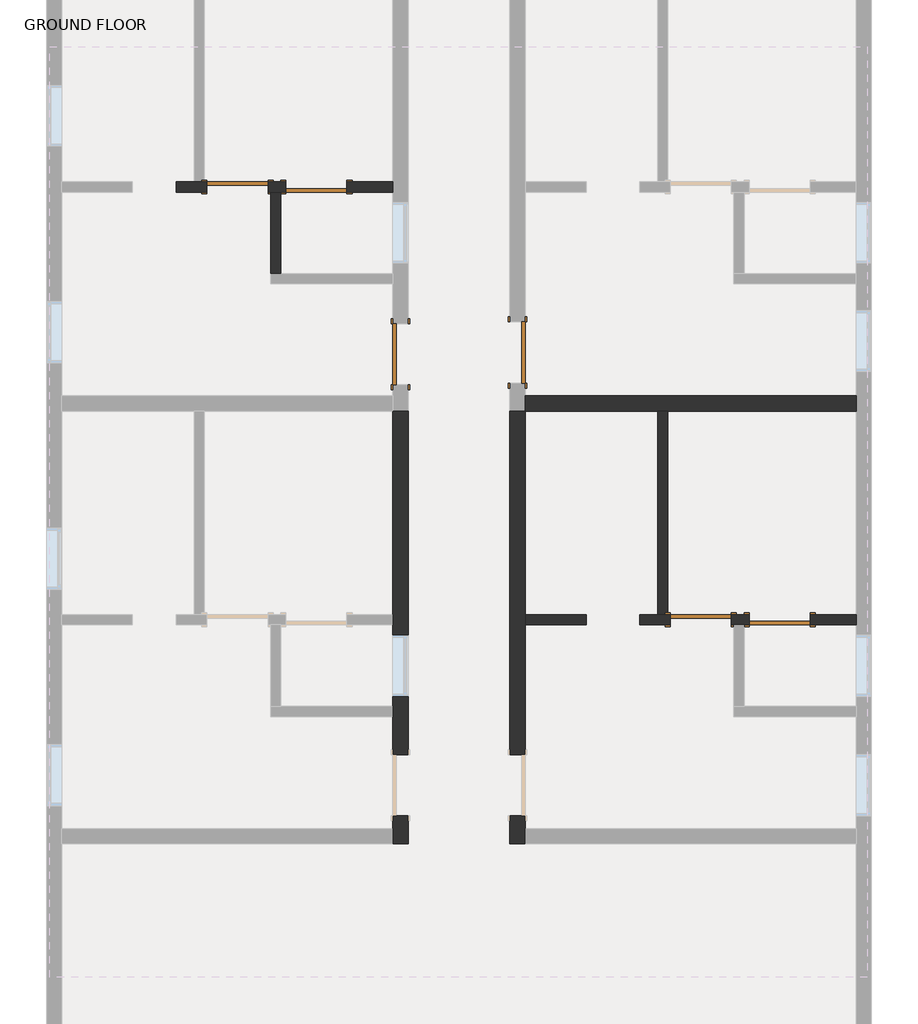
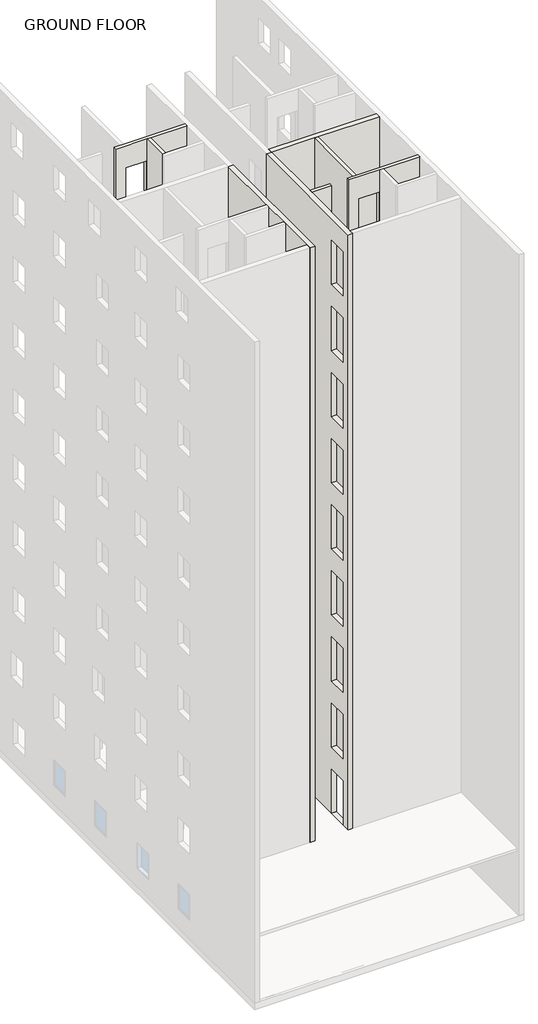
# One storey, part 3 of 7: 8 walls, 6 doors.
"""IFC4 building model written with IfcOpenShell, lengths in millimetres."""

from ifc_helpers import new_model, si_unit, origin, origin_with_axes, place, context, project, spatial, polyline, outline, extrude, faceted_brep, transform, mapped, element, save
from components import door_686f89d2, door_16372e1c, door_a90ba1ad, door_0ca8825f

model = new_model("IFC4")

# Units and contexts
model_context = context("Model", 3, world=origin())
ifc_project = project(units=[si_unit("LENGTHUNIT", "METRE", prefix="MILLI")], contexts=[model_context])

# Site, building, storey
site = spatial("IfcSite", under=ifc_project)
building = spatial("IfcBuilding", under=site)
storey = spatial("IfcBuildingStorey", under=building, Name="GROUND FLOOR", Elevation=0.0)

# Doors
placement = place(None, origin())
door_shape = door_686f89d2(model_context)
element("IfcDoor", 1, ObjectType="Single-Flush : 36\" x 84\"", at=placement, inside=storey, context=model_context, shape_type="MappedRepresentation", body=[
    mapped(door_shape, transform((-9863.5902461, -1001.7289408, 0.0), x_axis=(-1.0, 0.0, 0.0), y_axis=(0.0, -1.0, 0.0), z_axis=(0.0, 0.0, 1.0))),
])
element("IfcDoor", 2, ObjectType="Single-Flush : 36\" x 84\"", at=placement, inside=storey, context=model_context, shape_type="MappedRepresentation", body=[
    mapped(door_shape, transform((-2929.3902461, -7478.7289408, 0.0), x_axis=(-1.0, 0.0, 0.0), y_axis=(0.0, -1.0, 0.0), z_axis=(0.0, 0.0, 1.0))),
])
door_2_shape = door_16372e1c(model_context)
element("IfcDoor", 3, ObjectType="Single-Flush : 36\" x 84\"", at=placement, inside=storey, context=model_context, shape_type="MappedRepresentation", body=[
    mapped(door_2_shape, transform((-8682.4902461, -1001.7289408, 0.0), x_axis=(-1.0, 0.0, 0.0), y_axis=(0.0, -1.0, 0.0), z_axis=(0.0, 0.0, 1.0))),
])
element("IfcDoor", 4, ObjectType="Single-Flush : 36\" x 84\"", at=placement, inside=storey, context=model_context, shape_type="MappedRepresentation", body=[
    mapped(door_2_shape, transform((-1748.2902461, -7478.7289408, 0.0), x_axis=(-1.0, 0.0, 0.0), y_axis=(0.0, -1.0, 0.0), z_axis=(0.0, 0.0, 1.0))),
])
door_3_shape = door_a90ba1ad(model_context)
element("IfcDoor", 5, ObjectType="Single-Flush : 36\" x 84\"", at=placement, inside=storey, context=model_context, shape_type="MappedRepresentation", body=[
    mapped(door_3_shape, transform((-7425.1902461, -3503.6289408, 0.0), x_axis=(0.0, -1.0, 0.0), y_axis=(1.0, 0.0, 0.0), z_axis=(0.0, 0.0, 1.0))),
])
door_4_shape = door_0ca8825f(model_context)
element("IfcDoor", 6, ObjectType="Single-Flush : 36\" x 84\"", at=placement, inside=storey, context=model_context, shape_type="MappedRepresentation", body=[
    mapped(door_4_shape, transform((-5672.5902461, -3478.2289408, 0.0), x_axis=(0.0, -1.0, 0.0), y_axis=(1.0, 0.0, 0.0), z_axis=(0.0, 0.0, 1.0))),
])

# Walls
element("IfcWall", 7, ObjectType="Generic - 8\"", at=placement, inside=storey, context=model_context, shape_type="Brep", body=[
    faceted_brep([(-5558.2902461, -10831.5289408, 0.0), (-5558.2902461, -10602.9289408, 0.0), (-5558.2902461, -10412.4289408, 0.0), (-5558.2902461, -10412.4289408, 2133.6), (-5558.2902461, -9498.0289408, 2133.6), (-5558.2902461, -9498.0289408, 0.0), (-5558.2902461, -7554.9289408, 0.0), (-5558.2902461, -7402.5289408, 0.0), (-5558.2902461, -4354.5289408, 0.0), (-5558.2902461, -4354.5289408, 32004.0), (-5558.2902461, -7402.5289408, 32004.0), (-5558.2902461, -7554.9289408, 32004.0), (-5558.2902461, -10602.9289408, 32004.0), (-5558.2902461, -10831.5289408, 32004.0), (-5558.2902461, -9498.0289408, 3200.4), (-5558.2902461, -10412.4289408, 3200.4), (-5558.2902461, -10412.4289408, 5334.0), (-5558.2902461, -9498.0289408, 5334.0), (-5558.2902461, -9498.0289408, 6400.8), (-5558.2902461, -10412.4289408, 6400.8), (-5558.2902461, -10412.4289408, 8534.4), (-5558.2902461, -9498.0289408, 8534.4), (-5558.2902461, -9498.0289408, 9601.2), (-5558.2902461, -10412.4289408, 9601.2), (-5558.2902461, -10412.4289408, 11734.8), (-5558.2902461, -9498.0289408, 11734.8), (-5558.2902461, -9498.0289408, 12801.6), (-5558.2902461, -10412.4289408, 12801.6), (-5558.2902461, -10412.4289408, 14935.2), (-5558.2902461, -9498.0289408, 14935.2), (-5558.2902461, -9498.0289408, 16002.0), (-5558.2902461, -10412.4289408, 16002.0), (-5558.2902461, -10412.4289408, 18135.6), (-5558.2902461, -9498.0289408, 18135.6), (-5558.2902461, -9498.0289408, 19202.4), (-5558.2902461, -10412.4289408, 19202.4), (-5558.2902461, -10412.4289408, 21336.0), (-5558.2902461, -9498.0289408, 21336.0), (-5558.2902461, -9498.0289408, 22402.8), (-5558.2902461, -10412.4289408, 22402.8), (-5558.2902461, -10412.4289408, 24536.4), (-5558.2902461, -9498.0289408, 24536.4), (-5558.2902461, -9498.0289408, 25603.2), (-5558.2902461, -10412.4289408, 25603.2), (-5558.2902461, -10412.4289408, 27736.8), (-5558.2902461, -9498.0289408, 27736.8), (-5558.2902461, -9498.0289408, 28803.6), (-5558.2902461, -10412.4289408, 28803.6), (-5558.2902461, -10412.4289408, 30937.2), (-5558.2902461, -9498.0289408, 30937.2), (-5786.8902461, -10412.4289408, 2133.6), (-5786.8902461, -10412.4289408, 0.0), (-5786.8902461, -10831.5289408, 0.0), (-5786.8902461, -10831.5289408, 32004.0), (-5786.8902461, -4354.5289408, 32004.0), (-5786.8902461, -4354.5289408, 0.0), (-5786.8902461, -9498.0289408, 0.0), (-5786.8902461, -9498.0289408, 2133.6), (-5786.8902461, -9498.0289408, 3200.4), (-5786.8902461, -9498.0289408, 5334.0), (-5786.8902461, -10412.4289408, 5334.0), (-5786.8902461, -10412.4289408, 3200.4), (-5786.8902461, -9498.0289408, 6400.8), (-5786.8902461, -9498.0289408, 8534.4), (-5786.8902461, -10412.4289408, 8534.4), (-5786.8902461, -10412.4289408, 6400.8), (-5786.8902461, -9498.0289408, 9601.2), (-5786.8902461, -9498.0289408, 11734.8), (-5786.8902461, -10412.4289408, 11734.8), (-5786.8902461, -10412.4289408, 9601.2), (-5786.8902461, -9498.0289408, 12801.6), (-5786.8902461, -9498.0289408, 14935.2), (-5786.8902461, -10412.4289408, 14935.2), (-5786.8902461, -10412.4289408, 12801.6), (-5786.8902461, -9498.0289408, 16002.0), (-5786.8902461, -9498.0289408, 18135.6), (-5786.8902461, -10412.4289408, 18135.6), (-5786.8902461, -10412.4289408, 16002.0), (-5786.8902461, -9498.0289408, 19202.4), (-5786.8902461, -9498.0289408, 21336.0), (-5786.8902461, -10412.4289408, 21336.0), (-5786.8902461, -10412.4289408, 19202.4), (-5786.8902461, -9498.0289408, 22402.8), (-5786.8902461, -9498.0289408, 24536.4), (-5786.8902461, -10412.4289408, 24536.4), (-5786.8902461, -10412.4289408, 22402.8), (-5786.8902461, -9498.0289408, 25603.2), (-5786.8902461, -9498.0289408, 27736.8), (-5786.8902461, -10412.4289408, 27736.8), (-5786.8902461, -10412.4289408, 25603.2), (-5786.8902461, -9498.0289408, 28803.6), (-5786.8902461, -9498.0289408, 30937.2), (-5786.8902461, -10412.4289408, 30937.2), (-5786.8902461, -10412.4289408, 28803.6)], [[[0, 1, 2, 3, 4, 5, 6, 7, 8, 9, 10, 11, 12, 13], [14, 15, 16, 17], [18, 19, 20, 21], [22, 23, 24, 25], [26, 27, 28, 29], [30, 31, 32, 33], [34, 35, 36, 37], [38, 39, 40, 41], [42, 43, 44, 45], [46, 47, 48, 49]], [[50, 51, 52, 53, 54, 55, 56, 57], [58, 59, 60, 61], [62, 63, 64, 65], [66, 67, 68, 69], [70, 71, 72, 73], [74, 75, 76, 77], [78, 79, 80, 81], [82, 83, 84, 85], [86, 87, 88, 89], [90, 91, 92, 93]], [[56, 55, 8, 7, 6, 5]], [[52, 51, 2, 1, 0]], [[13, 12, 11, 10, 9, 54, 53]], [[0, 13, 53, 52]], [[9, 8, 55, 54]], [[3, 2, 51, 50]], [[4, 3, 50, 57]], [[5, 4, 57, 56]], [[15, 14, 58, 61]], [[16, 15, 61, 60]], [[17, 16, 60, 59]], [[14, 17, 59, 58]], [[19, 18, 62, 65]], [[20, 19, 65, 64]], [[21, 20, 64, 63]], [[18, 21, 63, 62]], [[23, 22, 66, 69]], [[24, 23, 69, 68]], [[25, 24, 68, 67]], [[22, 25, 67, 66]], [[27, 26, 70, 73]], [[28, 27, 73, 72]], [[29, 28, 72, 71]], [[26, 29, 71, 70]], [[31, 30, 74, 77]], [[32, 31, 77, 76]], [[33, 32, 76, 75]], [[30, 33, 75, 74]], [[35, 34, 78, 81]], [[36, 35, 81, 80]], [[37, 36, 80, 79]], [[34, 37, 79, 78]], [[39, 38, 82, 85]], [[40, 39, 85, 84]], [[41, 40, 84, 83]], [[38, 41, 83, 82]], [[43, 42, 86, 89]], [[44, 43, 89, 88]], [[45, 44, 88, 87]], [[42, 45, 87, 86]], [[47, 46, 90, 93]], [[48, 47, 93, 92]], [[49, 48, 92, 91]], [[46, 49, 91, 90]]]),
])
element("IfcWall", 8, ObjectType="INNER WALL 2", at=placement, inside=storey, context=model_context, shape_type="Brep", body=[
    faceted_brep([(-2472.1902461, -7554.9289408, 0.0), (-2434.0902461, -7554.9289408, 0.0), (-2281.6902461, -7554.9289408, 0.0), (-2205.4902461, -7554.9289408, 0.0), (-2205.4902461, -7554.9289408, 2133.6), (-1291.0902461, -7554.9289408, 2133.6), (-1291.0902461, -7554.9289408, 0.0), (-605.2902461, -7554.9289408, 0.0), (-605.2902461, -7554.9289408, 32004.0), (-2281.6902461, -7554.9289408, 32004.0), (-2434.0902461, -7554.9289408, 32004.0), (-3843.7902461, -7554.9289408, 32004.0), (-3843.7902461, -7554.9289408, 0.0), (-3386.5902461, -7554.9289408, 0.0), (-3386.5902461, -7554.9289408, 2133.6), (-2472.1902461, -7554.9289408, 2133.6), (-2472.1902461, -7554.9289408, 3200.4), (-3386.5902461, -7554.9289408, 3200.4), (-3386.5902461, -7554.9289408, 5334.0), (-2472.1902461, -7554.9289408, 5334.0), (-1291.0902461, -7554.9289408, 3200.4), (-2205.4902461, -7554.9289408, 3200.4), (-2205.4902461, -7554.9289408, 5334.0), (-1291.0902461, -7554.9289408, 5334.0), (-2472.1902461, -7554.9289408, 6400.8), (-3386.5902461, -7554.9289408, 6400.8), (-3386.5902461, -7554.9289408, 8534.4), (-2472.1902461, -7554.9289408, 8534.4), (-1291.0902461, -7554.9289408, 6400.8), (-2205.4902461, -7554.9289408, 6400.8), (-2205.4902461, -7554.9289408, 8534.4), (-1291.0902461, -7554.9289408, 8534.4), (-2472.1902461, -7554.9289408, 9601.2), (-3386.5902461, -7554.9289408, 9601.2), (-3386.5902461, -7554.9289408, 11734.8), (-2472.1902461, -7554.9289408, 11734.8), (-1291.0902461, -7554.9289408, 9601.2), (-2205.4902461, -7554.9289408, 9601.2), (-2205.4902461, -7554.9289408, 11734.8), (-1291.0902461, -7554.9289408, 11734.8), (-1291.0902461, -7554.9289408, 12801.6), (-2205.4902461, -7554.9289408, 12801.6), (-2205.4902461, -7554.9289408, 14935.2), (-1291.0902461, -7554.9289408, 14935.2), (-3386.5902461, -7554.9289408, 12801.6), (-3386.5902461, -7554.9289408, 14935.2), (-2472.1902461, -7554.9289408, 14935.2), (-2472.1902461, -7554.9289408, 12801.6), (-2472.1902461, -7554.9289408, 16002.0), (-3386.5902461, -7554.9289408, 16002.0), (-3386.5902461, -7554.9289408, 18135.6), (-2472.1902461, -7554.9289408, 18135.6), (-1291.0902461, -7554.9289408, 16002.0), (-2205.4902461, -7554.9289408, 16002.0), (-2205.4902461, -7554.9289408, 18135.6), (-1291.0902461, -7554.9289408, 18135.6), (-1291.0902461, -7554.9289408, 19202.4), (-2205.4902461, -7554.9289408, 19202.4), (-2205.4902461, -7554.9289408, 21336.0), (-1291.0902461, -7554.9289408, 21336.0), (-2472.1902461, -7554.9289408, 19202.4), (-3386.5902461, -7554.9289408, 19202.4), (-3386.5902461, -7554.9289408, 21336.0), (-2472.1902461, -7554.9289408, 21336.0), (-1291.0902461, -7554.9289408, 22402.8), (-2205.4902461, -7554.9289408, 22402.8), (-2205.4902461, -7554.9289408, 24536.4), (-1291.0902461, -7554.9289408, 24536.4), (-2472.1902461, -7554.9289408, 22402.8), (-3386.5902461, -7554.9289408, 22402.8), (-3386.5902461, -7554.9289408, 24536.4), (-2472.1902461, -7554.9289408, 24536.4), (-2472.1902461, -7554.9289408, 28803.6), (-3386.5902461, -7554.9289408, 28803.6), (-3386.5902461, -7554.9289408, 30937.2), (-2472.1902461, -7554.9289408, 30937.2), (-1291.0902461, -7554.9289408, 28803.6), (-2205.4902461, -7554.9289408, 28803.6), (-2205.4902461, -7554.9289408, 30937.2), (-1291.0902461, -7554.9289408, 30937.2), (-2205.4902461, -7402.5289408, 2133.6), (-2205.4902461, -7402.5289408, 0.0), (-2472.1902461, -7402.5289408, 0.0), (-2472.1902461, -7402.5289408, 2133.6), (-3386.5902461, -7402.5289408, 2133.6), (-3386.5902461, -7402.5289408, 0.0), (-3424.6902461, -7402.5289408, 0.0), (-3577.0902461, -7402.5289408, 0.0), (-3843.7902461, -7402.5289408, 0.0), (-3843.7902461, -7402.5289408, 32004.0), (-3577.0902461, -7402.5289408, 32004.0), (-3424.6902461, -7402.5289408, 32004.0), (-605.2902461, -7402.5289408, 32004.0), (-605.2902461, -7402.5289408, 0.0), (-1291.0902461, -7402.5289408, 0.0), (-1291.0902461, -7402.5289408, 2133.6), (-2472.1902461, -7402.5289408, 3200.4), (-2472.1902461, -7402.5289408, 5334.0), (-3386.5902461, -7402.5289408, 5334.0), (-3386.5902461, -7402.5289408, 3200.4), (-1291.0902461, -7402.5289408, 3200.4), (-1291.0902461, -7402.5289408, 5334.0), (-2205.4902461, -7402.5289408, 5334.0), (-2205.4902461, -7402.5289408, 3200.4), (-2472.1902461, -7402.5289408, 6400.8), (-2472.1902461, -7402.5289408, 8534.4), (-3386.5902461, -7402.5289408, 8534.4), (-3386.5902461, -7402.5289408, 6400.8), (-1291.0902461, -7402.5289408, 6400.8), (-1291.0902461, -7402.5289408, 8534.4), (-2205.4902461, -7402.5289408, 8534.4), (-2205.4902461, -7402.5289408, 6400.8), (-2472.1902461, -7402.5289408, 9601.2), (-2472.1902461, -7402.5289408, 11734.8), (-3386.5902461, -7402.5289408, 11734.8), (-3386.5902461, -7402.5289408, 9601.2), (-1291.0902461, -7402.5289408, 9601.2), (-1291.0902461, -7402.5289408, 11734.8), (-2205.4902461, -7402.5289408, 11734.8), (-2205.4902461, -7402.5289408, 9601.2), (-1291.0902461, -7402.5289408, 12801.6), (-1291.0902461, -7402.5289408, 14935.2), (-2205.4902461, -7402.5289408, 14935.2), (-2205.4902461, -7402.5289408, 12801.6), (-3386.5902461, -7402.5289408, 12801.6), (-2472.1902461, -7402.5289408, 12801.6), (-2472.1902461, -7402.5289408, 14935.2), (-3386.5902461, -7402.5289408, 14935.2), (-2472.1902461, -7402.5289408, 16002.0), (-2472.1902461, -7402.5289408, 18135.6), (-3386.5902461, -7402.5289408, 18135.6), (-3386.5902461, -7402.5289408, 16002.0), (-1291.0902461, -7402.5289408, 16002.0), (-1291.0902461, -7402.5289408, 18135.6), (-2205.4902461, -7402.5289408, 18135.6), (-2205.4902461, -7402.5289408, 16002.0), (-1291.0902461, -7402.5289408, 19202.4), (-1291.0902461, -7402.5289408, 21336.0), (-2205.4902461, -7402.5289408, 21336.0), (-2205.4902461, -7402.5289408, 19202.4), (-2472.1902461, -7402.5289408, 19202.4), (-2472.1902461, -7402.5289408, 21336.0), (-3386.5902461, -7402.5289408, 21336.0), (-3386.5902461, -7402.5289408, 19202.4), (-1291.0902461, -7402.5289408, 22402.8), (-1291.0902461, -7402.5289408, 24536.4), (-2205.4902461, -7402.5289408, 24536.4), (-2205.4902461, -7402.5289408, 22402.8), (-2472.1902461, -7402.5289408, 22402.8), (-2472.1902461, -7402.5289408, 24536.4), (-3386.5902461, -7402.5289408, 24536.4), (-3386.5902461, -7402.5289408, 22402.8), (-2472.1902461, -7402.5289408, 28803.6), (-2472.1902461, -7402.5289408, 30937.2), (-3386.5902461, -7402.5289408, 30937.2), (-3386.5902461, -7402.5289408, 28803.6), (-1291.0902461, -7402.5289408, 28803.6), (-1291.0902461, -7402.5289408, 30937.2), (-2205.4902461, -7402.5289408, 30937.2), (-2205.4902461, -7402.5289408, 28803.6)], [[[0, 1, 2, 3, 4, 5, 6, 7, 8, 9, 10, 11, 12, 13, 14, 15], [16, 17, 18, 19], [20, 21, 22, 23], [24, 25, 26, 27], [28, 29, 30, 31], [32, 33, 34, 35], [36, 37, 38, 39], [40, 41, 42, 43], [44, 45, 46, 47], [48, 49, 50, 51], [52, 53, 54, 55], [56, 57, 58, 59], [60, 61, 62, 63], [64, 65, 66, 67], [68, 69, 70, 71], [72, 73, 74, 75], [76, 77, 78, 79]], [[80, 81, 82, 83, 84, 85, 86, 87, 88, 89, 90, 91, 92, 93, 94, 95], [96, 97, 98, 99], [100, 101, 102, 103], [104, 105, 106, 107], [108, 109, 110, 111], [112, 113, 114, 115], [116, 117, 118, 119], [120, 121, 122, 123], [124, 125, 126, 127], [128, 129, 130, 131], [132, 133, 134, 135], [136, 137, 138, 139], [140, 141, 142, 143], [144, 145, 146, 147], [148, 149, 150, 151], [152, 153, 154, 155], [156, 157, 158, 159]], [[88, 87, 86, 85, 13, 12]], [[94, 93, 7, 6]], [[82, 81, 3, 2, 1, 0]], [[11, 10, 9, 8, 92, 91, 90, 89]], [[12, 11, 89, 88]], [[8, 7, 93, 92]], [[14, 13, 85, 84]], [[15, 14, 84, 83]], [[0, 15, 83, 82]], [[4, 3, 81, 80]], [[5, 4, 80, 95]], [[6, 5, 95, 94]], [[17, 16, 96, 99]], [[18, 17, 99, 98]], [[19, 18, 98, 97]], [[16, 19, 97, 96]], [[21, 20, 100, 103]], [[22, 21, 103, 102]], [[23, 22, 102, 101]], [[20, 23, 101, 100]], [[25, 24, 104, 107]], [[26, 25, 107, 106]], [[27, 26, 106, 105]], [[24, 27, 105, 104]], [[29, 28, 108, 111]], [[30, 29, 111, 110]], [[31, 30, 110, 109]], [[28, 31, 109, 108]], [[33, 32, 112, 115]], [[34, 33, 115, 114]], [[35, 34, 114, 113]], [[32, 35, 113, 112]], [[37, 36, 116, 119]], [[38, 37, 119, 118]], [[39, 38, 118, 117]], [[36, 39, 117, 116]], [[41, 40, 120, 123]], [[42, 41, 123, 122]], [[43, 42, 122, 121]], [[40, 43, 121, 120]], [[125, 124, 44, 47]], [[126, 125, 47, 46]], [[127, 126, 46, 45]], [[124, 127, 45, 44]], [[49, 48, 128, 131]], [[50, 49, 131, 130]], [[51, 50, 130, 129]], [[48, 51, 129, 128]], [[53, 52, 132, 135]], [[54, 53, 135, 134]], [[55, 54, 134, 133]], [[52, 55, 133, 132]], [[57, 56, 136, 139]], [[58, 57, 139, 138]], [[59, 58, 138, 137]], [[56, 59, 137, 136]], [[61, 60, 140, 143]], [[62, 61, 143, 142]], [[63, 62, 142, 141]], [[60, 63, 141, 140]], [[65, 64, 144, 147]], [[66, 65, 147, 146]], [[67, 66, 146, 145]], [[64, 67, 145, 144]], [[69, 68, 148, 151]], [[70, 69, 151, 150]], [[71, 70, 150, 149]], [[68, 71, 149, 148]], [[73, 72, 152, 155]], [[74, 73, 155, 154]], [[75, 74, 154, 153]], [[72, 75, 153, 152]], [[77, 76, 156, 159]], [[78, 77, 159, 158]], [[79, 78, 158, 157]], [[76, 79, 157, 156]]]),
])
element("IfcWall", 9, ObjectType="INNER WALL 2", at=placement, inside=storey, context=model_context, shape_type="SweptSolid", body=[
    extrude(outline(polyline([(-3424.6902461, -4354.5289408), (-3424.6902461, -7402.5289408), (-3577.0902461, -7402.5289408), (-3577.0902461, -4354.5289408), (-3424.6902461, -4354.5289408)])), origin_with_axes(), (0.0, 0.0, 1.0), 32004.0),
])
element("IfcWall", 10, ObjectType="INNER WALL 2", at=placement, inside=storey, context=model_context, shape_type="Brep", body=[
    faceted_brep([(-9406.3902461, -1077.9289408, 0.0), (-9368.2902461, -1077.9289408, 0.0), (-9215.8902461, -1077.9289408, 0.0), (-9139.6902461, -1077.9289408, 0.0), (-9139.6902461, -1077.9289408, 2133.6), (-8225.2902461, -1077.9289408, 2133.6), (-8225.2902461, -1077.9289408, 0.0), (-7539.4902461, -1077.9289408, 0.0), (-7539.4902461, -1077.9289408, 32004.0), (-9215.8902461, -1077.9289408, 32004.0), (-9368.2902461, -1077.9289408, 32004.0), (-10777.9902461, -1077.9289408, 32004.0), (-10777.9902461, -1077.9289408, 0.0), (-10320.7902461, -1077.9289408, 0.0), (-10320.7902461, -1077.9289408, 2133.6), (-9406.3902461, -1077.9289408, 2133.6), (-9406.3902461, -1077.9289408, 3200.4), (-10320.7902461, -1077.9289408, 3200.4), (-10320.7902461, -1077.9289408, 5334.0), (-9406.3902461, -1077.9289408, 5334.0), (-8225.2902461, -1077.9289408, 3200.4), (-9139.6902461, -1077.9289408, 3200.4), (-9139.6902461, -1077.9289408, 5334.0), (-8225.2902461, -1077.9289408, 5334.0), (-8225.2902461, -1077.9289408, 6400.8), (-9139.6902461, -1077.9289408, 6400.8), (-9139.6902461, -1077.9289408, 8534.4), (-8225.2902461, -1077.9289408, 8534.4), (-9406.3902461, -1077.9289408, 6400.8), (-10320.7902461, -1077.9289408, 6400.8), (-10320.7902461, -1077.9289408, 8534.4), (-9406.3902461, -1077.9289408, 8534.4), (-9406.3902461, -1077.9289408, 9601.2), (-10320.7902461, -1077.9289408, 9601.2), (-10320.7902461, -1077.9289408, 11734.8), (-9406.3902461, -1077.9289408, 11734.8), (-8225.2902461, -1077.9289408, 9601.2), (-9139.6902461, -1077.9289408, 9601.2), (-9139.6902461, -1077.9289408, 11734.8), (-8225.2902461, -1077.9289408, 11734.8), (-9406.3902461, -1077.9289408, 12801.6), (-10320.7902461, -1077.9289408, 12801.6), (-10320.7902461, -1077.9289408, 14935.2), (-9406.3902461, -1077.9289408, 14935.2), (-8225.2902461, -1077.9289408, 12801.6), (-9139.6902461, -1077.9289408, 12801.6), (-9139.6902461, -1077.9289408, 14935.2), (-8225.2902461, -1077.9289408, 14935.2), (-9406.3902461, -1077.9289408, 16002.0), (-10320.7902461, -1077.9289408, 16002.0), (-10320.7902461, -1077.9289408, 18135.6), (-9406.3902461, -1077.9289408, 18135.6), (-8225.2902461, -1077.9289408, 16002.0), (-9139.6902461, -1077.9289408, 16002.0), (-9139.6902461, -1077.9289408, 18135.6), (-8225.2902461, -1077.9289408, 18135.6), (-9406.3902461, -1077.9289408, 19202.4), (-10320.7902461, -1077.9289408, 19202.4), (-10320.7902461, -1077.9289408, 21336.0), (-9406.3902461, -1077.9289408, 21336.0), (-8225.2902461, -1077.9289408, 19202.4), (-9139.6902461, -1077.9289408, 19202.4), (-9139.6902461, -1077.9289408, 21336.0), (-8225.2902461, -1077.9289408, 21336.0), (-9406.3902461, -1077.9289408, 22402.8), (-10320.7902461, -1077.9289408, 22402.8), (-10320.7902461, -1077.9289408, 24536.4), (-9406.3902461, -1077.9289408, 24536.4), (-8225.2902461, -1077.9289408, 22402.8), (-9139.6902461, -1077.9289408, 22402.8), (-9139.6902461, -1077.9289408, 24536.4), (-8225.2902461, -1077.9289408, 24536.4), (-8225.2902461, -1077.9289408, 25603.2), (-9139.6902461, -1077.9289408, 25603.2), (-9139.6902461, -1077.9289408, 27736.8), (-8225.2902461, -1077.9289408, 27736.8), (-9406.3902461, -1077.9289408, 25603.2), (-10320.7902461, -1077.9289408, 25603.2), (-10320.7902461, -1077.9289408, 27736.8), (-9406.3902461, -1077.9289408, 27736.8), (-9406.3902461, -1077.9289408, 28803.6), (-10320.7902461, -1077.9289408, 28803.6), (-10320.7902461, -1077.9289408, 30937.2), (-9406.3902461, -1077.9289408, 30937.2), (-8225.2902461, -1077.9289408, 28803.6), (-9139.6902461, -1077.9289408, 28803.6), (-9139.6902461, -1077.9289408, 30937.2), (-8225.2902461, -1077.9289408, 30937.2), (-9139.6902461, -925.5289408, 2133.6), (-9139.6902461, -925.5289408, 0.0), (-9406.3902461, -925.5289408, 0.0), (-9406.3902461, -925.5289408, 2133.6), (-10320.7902461, -925.5289408, 2133.6), (-10320.7902461, -925.5289408, 0.0), (-10358.8902461, -925.5289408, 0.0), (-10511.2902461, -925.5289408, 0.0), (-10777.9902461, -925.5289408, 0.0), (-10777.9902461, -925.5289408, 32004.0), (-10511.2902461, -925.5289408, 32004.0), (-10358.8902461, -925.5289408, 32004.0), (-7539.4902461, -925.5289408, 32004.0), (-7539.4902461, -925.5289408, 0.0), (-8225.2902461, -925.5289408, 0.0), (-8225.2902461, -925.5289408, 2133.6), (-9406.3902461, -925.5289408, 3200.4), (-9406.3902461, -925.5289408, 5334.0), (-10320.7902461, -925.5289408, 5334.0), (-10320.7902461, -925.5289408, 3200.4), (-8225.2902461, -925.5289408, 3200.4), (-8225.2902461, -925.5289408, 5334.0), (-9139.6902461, -925.5289408, 5334.0), (-9139.6902461, -925.5289408, 3200.4), (-8225.2902461, -925.5289408, 6400.8), (-8225.2902461, -925.5289408, 8534.4), (-9139.6902461, -925.5289408, 8534.4), (-9139.6902461, -925.5289408, 6400.8), (-9406.3902461, -925.5289408, 6400.8), (-9406.3902461, -925.5289408, 8534.4), (-10320.7902461, -925.5289408, 8534.4), (-10320.7902461, -925.5289408, 6400.8), (-9406.3902461, -925.5289408, 9601.2), (-9406.3902461, -925.5289408, 11734.8), (-10320.7902461, -925.5289408, 11734.8), (-10320.7902461, -925.5289408, 9601.2), (-8225.2902461, -925.5289408, 9601.2), (-8225.2902461, -925.5289408, 11734.8), (-9139.6902461, -925.5289408, 11734.8), (-9139.6902461, -925.5289408, 9601.2), (-9406.3902461, -925.5289408, 12801.6), (-9406.3902461, -925.5289408, 14935.2), (-10320.7902461, -925.5289408, 14935.2), (-10320.7902461, -925.5289408, 12801.6), (-8225.2902461, -925.5289408, 12801.6), (-8225.2902461, -925.5289408, 14935.2), (-9139.6902461, -925.5289408, 14935.2), (-9139.6902461, -925.5289408, 12801.6), (-9406.3902461, -925.5289408, 16002.0), (-9406.3902461, -925.5289408, 18135.6), (-10320.7902461, -925.5289408, 18135.6), (-10320.7902461, -925.5289408, 16002.0), (-8225.2902461, -925.5289408, 16002.0), (-8225.2902461, -925.5289408, 18135.6), (-9139.6902461, -925.5289408, 18135.6), (-9139.6902461, -925.5289408, 16002.0), (-9406.3902461, -925.5289408, 19202.4), (-9406.3902461, -925.5289408, 21336.0), (-10320.7902461, -925.5289408, 21336.0), (-10320.7902461, -925.5289408, 19202.4), (-8225.2902461, -925.5289408, 19202.4), (-8225.2902461, -925.5289408, 21336.0), (-9139.6902461, -925.5289408, 21336.0), (-9139.6902461, -925.5289408, 19202.4), (-9406.3902461, -925.5289408, 22402.8), (-9406.3902461, -925.5289408, 24536.4), (-10320.7902461, -925.5289408, 24536.4), (-10320.7902461, -925.5289408, 22402.8), (-8225.2902461, -925.5289408, 22402.8), (-8225.2902461, -925.5289408, 24536.4), (-9139.6902461, -925.5289408, 24536.4), (-9139.6902461, -925.5289408, 22402.8), (-8225.2902461, -925.5289408, 25603.2), (-8225.2902461, -925.5289408, 27736.8), (-9139.6902461, -925.5289408, 27736.8), (-9139.6902461, -925.5289408, 25603.2), (-9406.3902461, -925.5289408, 25603.2), (-9406.3902461, -925.5289408, 27736.8), (-10320.7902461, -925.5289408, 27736.8), (-10320.7902461, -925.5289408, 25603.2), (-9406.3902461, -925.5289408, 28803.6), (-9406.3902461, -925.5289408, 30937.2), (-10320.7902461, -925.5289408, 30937.2), (-10320.7902461, -925.5289408, 28803.6), (-8225.2902461, -925.5289408, 28803.6), (-8225.2902461, -925.5289408, 30937.2), (-9139.6902461, -925.5289408, 30937.2), (-9139.6902461, -925.5289408, 28803.6)], [[[0, 1, 2, 3, 4, 5, 6, 7, 8, 9, 10, 11, 12, 13, 14, 15], [16, 17, 18, 19], [20, 21, 22, 23], [24, 25, 26, 27], [28, 29, 30, 31], [32, 33, 34, 35], [36, 37, 38, 39], [40, 41, 42, 43], [44, 45, 46, 47], [48, 49, 50, 51], [52, 53, 54, 55], [56, 57, 58, 59], [60, 61, 62, 63], [64, 65, 66, 67], [68, 69, 70, 71], [72, 73, 74, 75], [76, 77, 78, 79], [80, 81, 82, 83], [84, 85, 86, 87]], [[88, 89, 90, 91, 92, 93, 94, 95, 96, 97, 98, 99, 100, 101, 102, 103], [104, 105, 106, 107], [108, 109, 110, 111], [112, 113, 114, 115], [116, 117, 118, 119], [120, 121, 122, 123], [124, 125, 126, 127], [128, 129, 130, 131], [132, 133, 134, 135], [136, 137, 138, 139], [140, 141, 142, 143], [144, 145, 146, 147], [148, 149, 150, 151], [152, 153, 154, 155], [156, 157, 158, 159], [160, 161, 162, 163], [164, 165, 166, 167], [168, 169, 170, 171], [172, 173, 174, 175]], [[96, 95, 94, 93, 13, 12]], [[102, 101, 7, 6]], [[90, 89, 3, 2, 1, 0]], [[11, 10, 9, 8, 100, 99, 98, 97]], [[12, 11, 97, 96]], [[8, 7, 101, 100]], [[14, 13, 93, 92]], [[15, 14, 92, 91]], [[0, 15, 91, 90]], [[4, 3, 89, 88]], [[5, 4, 88, 103]], [[6, 5, 103, 102]], [[17, 16, 104, 107]], [[18, 17, 107, 106]], [[19, 18, 106, 105]], [[16, 19, 105, 104]], [[21, 20, 108, 111]], [[22, 21, 111, 110]], [[23, 22, 110, 109]], [[20, 23, 109, 108]], [[25, 24, 112, 115]], [[26, 25, 115, 114]], [[27, 26, 114, 113]], [[24, 27, 113, 112]], [[29, 28, 116, 119]], [[30, 29, 119, 118]], [[31, 30, 118, 117]], [[28, 31, 117, 116]], [[33, 32, 120, 123]], [[34, 33, 123, 122]], [[35, 34, 122, 121]], [[32, 35, 121, 120]], [[37, 36, 124, 127]], [[38, 37, 127, 126]], [[39, 38, 126, 125]], [[36, 39, 125, 124]], [[41, 40, 128, 131]], [[42, 41, 131, 130]], [[43, 42, 130, 129]], [[40, 43, 129, 128]], [[45, 44, 132, 135]], [[46, 45, 135, 134]], [[47, 46, 134, 133]], [[44, 47, 133, 132]], [[49, 48, 136, 139]], [[50, 49, 139, 138]], [[51, 50, 138, 137]], [[48, 51, 137, 136]], [[53, 52, 140, 143]], [[54, 53, 143, 142]], [[55, 54, 142, 141]], [[52, 55, 141, 140]], [[57, 56, 144, 147]], [[58, 57, 147, 146]], [[59, 58, 146, 145]], [[56, 59, 145, 144]], [[61, 60, 148, 151]], [[62, 61, 151, 150]], [[63, 62, 150, 149]], [[60, 63, 149, 148]], [[65, 64, 152, 155]], [[66, 65, 155, 154]], [[67, 66, 154, 153]], [[64, 67, 153, 152]], [[69, 68, 156, 159]], [[70, 69, 159, 158]], [[71, 70, 158, 157]], [[68, 71, 157, 156]], [[73, 72, 160, 163]], [[74, 73, 163, 162]], [[75, 74, 162, 161]], [[72, 75, 161, 160]], [[77, 76, 164, 167]], [[78, 77, 167, 166]], [[79, 78, 166, 165]], [[76, 79, 165, 164]], [[81, 80, 168, 171]], [[82, 81, 171, 170]], [[83, 82, 170, 169]], [[80, 83, 169, 168]], [[85, 84, 172, 175]], [[86, 85, 175, 174]], [[87, 86, 174, 173]], [[84, 87, 173, 172]]]),
])
element("IfcWall", 11, ObjectType="INNER WALL 2", at=placement, inside=storey, context=model_context, shape_type="SweptSolid", body=[
    extrude(outline(polyline([(-9215.8902461, -1077.9289408), (-9215.8902461, -2297.1289408), (-9368.2902461, -2297.1289408), (-9368.2902461, -1077.9289408), (-9215.8902461, -1077.9289408)])), origin_with_axes(), (0.0, 0.0, 1.0), 32004.0),
])
element("IfcWall", 12, ObjectType="INNER WALL 2", at=placement, inside=storey, context=model_context, shape_type="SweptSolid", body=[
    extrude(outline(polyline([(-4643.8902461, -7554.9289408), (-5558.2902461, -7554.9289408), (-5558.2902461, -7402.5289408), (-4643.8902461, -7402.5289408), (-4643.8902461, -7554.9289408)])), origin_with_axes(), (0.0, 0.0, 1.0), 32004.0),
])
element("IfcWall", 13, ObjectType="OUTER WALL", at=placement, inside=storey, context=model_context, shape_type="Brep", body=[
    faceted_brep([(-605.2902461, -4125.9289408, 0.0), (-5558.2902461, -4125.9289408, 0.0), (-5558.2902461, -4125.9289408, 32004.0), (-605.2902461, -4125.9289408, 32004.0), (-605.2902461, -4354.5289408, 0.0), (-605.2902461, -4354.5289408, 32004.0), (-3424.6902461, -4354.5289408, 32004.0), (-3577.0902461, -4354.5289408, 32004.0), (-5558.2902461, -4354.5289408, 32004.0), (-5558.2902461, -4354.5289408, 0.0), (-3577.0902461, -4354.5289408, 0.0), (-3424.6902461, -4354.5289408, 0.0)], [[[0, 1, 2, 3]], [[4, 5, 6, 7, 8, 9, 10, 11]], [[1, 0, 4, 11, 10, 9]], [[3, 2, 8, 7, 6, 5]], [[2, 1, 9, 8]], [[0, 3, 5, 4]]]),
])
element("IfcWall", 14, ObjectType="OUTER WALL", at=placement, inside=storey, context=model_context, shape_type="Brep", body=[
    faceted_brep([(-7310.8902461, -10831.5289408, 0.0), (-7310.8902461, -10412.4289408, 0.0), (-7310.8902461, -10412.4289408, 2133.6), (-7310.8902461, -9498.0289408, 2133.6), (-7310.8902461, -9498.0289408, 0.0), (-7310.8902461, -4354.5289408, 0.0), (-7310.8902461, -4354.5289408, 32004.0), (-7310.8902461, -10831.5289408, 32004.0), (-7310.8902461, -8621.7289408, 2133.6), (-7310.8902461, -7707.3289408, 2133.6), (-7310.8902461, -7707.3289408, 914.4), (-7310.8902461, -8621.7289408, 914.4), (-7310.8902461, -9498.0289408, 3200.4), (-7310.8902461, -10412.4289408, 3200.4), (-7310.8902461, -10412.4289408, 5334.0), (-7310.8902461, -9498.0289408, 5334.0), (-7310.8902461, -8621.7289408, 5334.0), (-7310.8902461, -7707.3289408, 5334.0), (-7310.8902461, -7707.3289408, 4114.8), (-7310.8902461, -8621.7289408, 4114.8), (-7310.8902461, -9498.0289408, 6400.8), (-7310.8902461, -10412.4289408, 6400.8), (-7310.8902461, -10412.4289408, 8534.4), (-7310.8902461, -9498.0289408, 8534.4), (-7310.8902461, -8621.7289408, 8534.4), (-7310.8902461, -7707.3289408, 8534.4), (-7310.8902461, -7707.3289408, 7315.2), (-7310.8902461, -8621.7289408, 7315.2), (-7310.8902461, -9498.0289408, 9601.2), (-7310.8902461, -10412.4289408, 9601.2), (-7310.8902461, -10412.4289408, 11734.8), (-7310.8902461, -9498.0289408, 11734.8), (-7310.8902461, -8621.7289408, 11734.8), (-7310.8902461, -7707.3289408, 11734.8), (-7310.8902461, -7707.3289408, 10515.6), (-7310.8902461, -8621.7289408, 10515.6), (-7310.8902461, -9498.0289408, 12801.6), (-7310.8902461, -10412.4289408, 12801.6), (-7310.8902461, -10412.4289408, 14935.2), (-7310.8902461, -9498.0289408, 14935.2), (-7310.8902461, -8621.7289408, 14935.2), (-7310.8902461, -7707.3289408, 14935.2), (-7310.8902461, -7707.3289408, 13716.0), (-7310.8902461, -8621.7289408, 13716.0), (-7310.8902461, -9498.0289408, 16002.0), (-7310.8902461, -10412.4289408, 16002.0), (-7310.8902461, -10412.4289408, 18135.6), (-7310.8902461, -9498.0289408, 18135.6), (-7310.8902461, -8621.7289408, 18135.6), (-7310.8902461, -7707.3289408, 18135.6), (-7310.8902461, -7707.3289408, 16916.4), (-7310.8902461, -8621.7289408, 16916.4), (-7310.8902461, -9498.0289408, 19202.4), (-7310.8902461, -10412.4289408, 19202.4), (-7310.8902461, -10412.4289408, 21336.0), (-7310.8902461, -9498.0289408, 21336.0), (-7310.8902461, -8621.7289408, 21336.0), (-7310.8902461, -7707.3289408, 21336.0), (-7310.8902461, -7707.3289408, 20116.8), (-7310.8902461, -8621.7289408, 20116.8), (-7310.8902461, -9498.0289408, 22402.8), (-7310.8902461, -10412.4289408, 22402.8), (-7310.8902461, -10412.4289408, 24536.4), (-7310.8902461, -9498.0289408, 24536.4), (-7310.8902461, -8621.7289408, 24536.4), (-7310.8902461, -7707.3289408, 24536.4), (-7310.8902461, -7707.3289408, 23317.2), (-7310.8902461, -8621.7289408, 23317.2), (-7310.8902461, -9498.0289408, 25603.2), (-7310.8902461, -10412.4289408, 25603.2), (-7310.8902461, -10412.4289408, 27736.8), (-7310.8902461, -9498.0289408, 27736.8), (-7310.8902461, -8621.7289408, 27736.8), (-7310.8902461, -7707.3289408, 27736.8), (-7310.8902461, -7707.3289408, 26517.6), (-7310.8902461, -8621.7289408, 26517.6), (-7310.8902461, -9498.0289408, 28803.6), (-7310.8902461, -10412.4289408, 28803.6), (-7310.8902461, -10412.4289408, 30937.2), (-7310.8902461, -9498.0289408, 30937.2), (-7310.8902461, -8621.7289408, 30937.2), (-7310.8902461, -7707.3289408, 30937.2), (-7310.8902461, -7707.3289408, 29718.0), (-7310.8902461, -8621.7289408, 29718.0), (-7539.4902461, -10412.4289408, 2133.6), (-7539.4902461, -10412.4289408, 0.0), (-7539.4902461, -10602.9289408, 0.0), (-7539.4902461, -10831.5289408, 0.0), (-7539.4902461, -10831.5289408, 32004.0), (-7539.4902461, -10602.9289408, 32004.0), (-7539.4902461, -8926.5289408, 32004.0), (-7539.4902461, -8774.1289408, 32004.0), (-7539.4902461, -7554.9289408, 32004.0), (-7539.4902461, -7402.5289408, 32004.0), (-7539.4902461, -4354.5289408, 32004.0), (-7539.4902461, -4354.5289408, 0.0), (-7539.4902461, -7402.5289408, 0.0), (-7539.4902461, -7554.9289408, 0.0), (-7539.4902461, -8774.1289408, 0.0), (-7539.4902461, -8926.5289408, 0.0), (-7539.4902461, -9498.0289408, 0.0), (-7539.4902461, -9498.0289408, 2133.6), (-7539.4902461, -8621.7289408, 2133.6), (-7539.4902461, -8621.7289408, 914.4), (-7539.4902461, -7707.3289408, 914.4), (-7539.4902461, -7707.3289408, 2133.6), (-7539.4902461, -9498.0289408, 3200.4), (-7539.4902461, -9498.0289408, 5334.0), (-7539.4902461, -10412.4289408, 5334.0), (-7539.4902461, -10412.4289408, 3200.4), (-7539.4902461, -8621.7289408, 5334.0), (-7539.4902461, -8621.7289408, 4114.8), (-7539.4902461, -7707.3289408, 4114.8), (-7539.4902461, -7707.3289408, 5334.0), (-7539.4902461, -9498.0289408, 6400.8), (-7539.4902461, -9498.0289408, 8534.4), (-7539.4902461, -10412.4289408, 8534.4), (-7539.4902461, -10412.4289408, 6400.8), (-7539.4902461, -8621.7289408, 8534.4), (-7539.4902461, -8621.7289408, 7315.2), (-7539.4902461, -7707.3289408, 7315.2), (-7539.4902461, -7707.3289408, 8534.4), (-7539.4902461, -9498.0289408, 9601.2), (-7539.4902461, -9498.0289408, 11734.8), (-7539.4902461, -10412.4289408, 11734.8), (-7539.4902461, -10412.4289408, 9601.2), (-7539.4902461, -8621.7289408, 11734.8), (-7539.4902461, -8621.7289408, 10515.6), (-7539.4902461, -7707.3289408, 10515.6), (-7539.4902461, -7707.3289408, 11734.8), (-7539.4902461, -9498.0289408, 12801.6), (-7539.4902461, -9498.0289408, 14935.2), (-7539.4902461, -10412.4289408, 14935.2), (-7539.4902461, -10412.4289408, 12801.6), (-7539.4902461, -8621.7289408, 14935.2), (-7539.4902461, -8621.7289408, 13716.0), (-7539.4902461, -7707.3289408, 13716.0), (-7539.4902461, -7707.3289408, 14935.2), (-7539.4902461, -9498.0289408, 16002.0), (-7539.4902461, -9498.0289408, 18135.6), (-7539.4902461, -10412.4289408, 18135.6), (-7539.4902461, -10412.4289408, 16002.0), (-7539.4902461, -8621.7289408, 18135.6), (-7539.4902461, -8621.7289408, 16916.4), (-7539.4902461, -7707.3289408, 16916.4), (-7539.4902461, -7707.3289408, 18135.6), (-7539.4902461, -9498.0289408, 19202.4), (-7539.4902461, -9498.0289408, 21336.0), (-7539.4902461, -10412.4289408, 21336.0), (-7539.4902461, -10412.4289408, 19202.4), (-7539.4902461, -8621.7289408, 21336.0), (-7539.4902461, -8621.7289408, 20116.8), (-7539.4902461, -7707.3289408, 20116.8), (-7539.4902461, -7707.3289408, 21336.0), (-7539.4902461, -9498.0289408, 22402.8), (-7539.4902461, -9498.0289408, 24536.4), (-7539.4902461, -10412.4289408, 24536.4), (-7539.4902461, -10412.4289408, 22402.8), (-7539.4902461, -8621.7289408, 24536.4), (-7539.4902461, -8621.7289408, 23317.2), (-7539.4902461, -7707.3289408, 23317.2), (-7539.4902461, -7707.3289408, 24536.4), (-7539.4902461, -9498.0289408, 25603.2), (-7539.4902461, -9498.0289408, 27736.8), (-7539.4902461, -10412.4289408, 27736.8), (-7539.4902461, -10412.4289408, 25603.2), (-7539.4902461, -8621.7289408, 27736.8), (-7539.4902461, -8621.7289408, 26517.6), (-7539.4902461, -7707.3289408, 26517.6), (-7539.4902461, -7707.3289408, 27736.8), (-7539.4902461, -9498.0289408, 28803.6), (-7539.4902461, -9498.0289408, 30937.2), (-7539.4902461, -10412.4289408, 30937.2), (-7539.4902461, -10412.4289408, 28803.6), (-7539.4902461, -8621.7289408, 30937.2), (-7539.4902461, -8621.7289408, 29718.0), (-7539.4902461, -7707.3289408, 29718.0), (-7539.4902461, -7707.3289408, 30937.2)], [[[0, 1, 2, 3, 4, 5, 6, 7], [8, 9, 10, 11], [12, 13, 14, 15], [16, 17, 18, 19], [20, 21, 22, 23], [24, 25, 26, 27], [28, 29, 30, 31], [32, 33, 34, 35], [36, 37, 38, 39], [40, 41, 42, 43], [44, 45, 46, 47], [48, 49, 50, 51], [52, 53, 54, 55], [56, 57, 58, 59], [60, 61, 62, 63], [64, 65, 66, 67], [68, 69, 70, 71], [72, 73, 74, 75], [76, 77, 78, 79], [80, 81, 82, 83]], [[84, 85, 86, 87, 88, 89, 90, 91, 92, 93, 94, 95, 96, 97, 98, 99, 100, 101], [102, 103, 104, 105], [106, 107, 108, 109], [110, 111, 112, 113], [114, 115, 116, 117], [118, 119, 120, 121], [122, 123, 124, 125], [126, 127, 128, 129], [130, 131, 132, 133], [134, 135, 136, 137], [138, 139, 140, 141], [142, 143, 144, 145], [146, 147, 148, 149], [150, 151, 152, 153], [154, 155, 156, 157], [158, 159, 160, 161], [162, 163, 164, 165], [166, 167, 168, 169], [170, 171, 172, 173], [174, 175, 176, 177]], [[87, 86, 85, 1, 0]], [[100, 99, 98, 97, 96, 95, 5, 4]], [[7, 6, 94, 93, 92, 91, 90, 89, 88]], [[0, 7, 88, 87]], [[6, 5, 95, 94]], [[2, 1, 85, 84]], [[3, 2, 84, 101]], [[4, 3, 101, 100]], [[103, 102, 8, 11]], [[104, 103, 11, 10]], [[105, 104, 10, 9]], [[102, 105, 9, 8]], [[13, 12, 106, 109]], [[14, 13, 109, 108]], [[15, 14, 108, 107]], [[12, 15, 107, 106]], [[111, 110, 16, 19]], [[112, 111, 19, 18]], [[113, 112, 18, 17]], [[110, 113, 17, 16]], [[21, 20, 114, 117]], [[22, 21, 117, 116]], [[23, 22, 116, 115]], [[20, 23, 115, 114]], [[119, 118, 24, 27]], [[120, 119, 27, 26]], [[121, 120, 26, 25]], [[118, 121, 25, 24]], [[29, 28, 122, 125]], [[30, 29, 125, 124]], [[31, 30, 124, 123]], [[28, 31, 123, 122]], [[127, 126, 32, 35]], [[128, 127, 35, 34]], [[129, 128, 34, 33]], [[126, 129, 33, 32]], [[37, 36, 130, 133]], [[38, 37, 133, 132]], [[39, 38, 132, 131]], [[36, 39, 131, 130]], [[135, 134, 40, 43]], [[136, 135, 43, 42]], [[137, 136, 42, 41]], [[134, 137, 41, 40]], [[45, 44, 138, 141]], [[46, 45, 141, 140]], [[47, 46, 140, 139]], [[44, 47, 139, 138]], [[143, 142, 48, 51]], [[144, 143, 51, 50]], [[145, 144, 50, 49]], [[142, 145, 49, 48]], [[53, 52, 146, 149]], [[54, 53, 149, 148]], [[55, 54, 148, 147]], [[52, 55, 147, 146]], [[151, 150, 56, 59]], [[152, 151, 59, 58]], [[153, 152, 58, 57]], [[150, 153, 57, 56]], [[61, 60, 154, 157]], [[62, 61, 157, 156]], [[63, 62, 156, 155]], [[60, 63, 155, 154]], [[159, 158, 64, 67]], [[160, 159, 67, 66]], [[161, 160, 66, 65]], [[158, 161, 65, 64]], [[69, 68, 162, 165]], [[70, 69, 165, 164]], [[71, 70, 164, 163]], [[68, 71, 163, 162]], [[167, 166, 72, 75]], [[168, 167, 75, 74]], [[169, 168, 74, 73]], [[166, 169, 73, 72]], [[77, 76, 170, 173]], [[78, 77, 173, 172]], [[79, 78, 172, 171]], [[76, 79, 171, 170]], [[175, 174, 80, 83]], [[176, 175, 83, 82]], [[177, 176, 82, 81]], [[174, 177, 81, 80]]]),
])

save(model, "model.ifc")

# Revit data of these elements
# Type "Single-Flush : 36\" x 84\""
#   Type Mark = "1"
#   Construction Type Id = "MDOOR"
#   Assembly Code = "C1020"
#   Analytic Construction = "Metal"
#   Thickness = 0' - 2"
#   Heat Transfer Coefficient (U) = 0.651978 BTU/(h·ft²·°F)
#   Height = 7' - 0"
#   Trim Projection Ext = 0' - 1"
#   Trim Projection Int = 0' - 1"
#   Trim Width = 0' - 3"
#   Width = 3' - 0"
#   Define Thermal Properties by = 1
#   Door Material = Door - Panel
#   Frame Material = Door - Frame
#   Visual Light Transmittance = 0
#   Solar Heat Gain Coefficient = 0
#   Function = (empty or 0)
#   Wall Closure = (empty or 0)
# Type "Generic - 8\""
#   Assembly Code = "B2010"
#   Layers, outside or top first: 0' - 9" no material (function 1)
# Type "INNER WALL 2"
#   Assembly Code = "B2010"
#   Layers, outside or top first: 0' - 6" no material (function 1)
# Type "OUTER WALL"
#   Assembly Code = "B2010"
#   Layers, outside or top first: 0' - 9" no material (function 1)
# Elements 1, 2, 3, 4, 5, 6 (IfcDoor, "Single-Flush : 36\" x 84\"")
#   Phase Created = New Construction
#   Materials on its faces: "Door - Frame", "Door - Panel"
# Element 7 (IfcWall, "Generic - 8\"")
#   Top Offset = 0' - 0"
#   Base Offset = 0' - 0"
#   Unconnected Height = 105' - 0"
#   wall height = 105' - 0"
#   Phase Created = New Construction
#   Base Constraint = GROUND FLOOR
#   Materials on its faces: "Default Wall"
# Elements 8, 9, 10, 11, 12 (IfcWall, "INNER WALL 2")
#   Top Offset = 0' - 0"
#   Base Offset = 0' - 0"
#   Unconnected Height = 105' - 0"
#   wall height = 105' - 0"
#   Phase Created = New Construction
#   Base Constraint = GROUND FLOOR
#   Materials on its faces: "Default Wall"
# Elements 13, 14 (IfcWall, "OUTER WALL")
#   Top Offset = 0' - 0"
#   Base Offset = 0' - 0"
#   Unconnected Height = 105' - 0"
#   wall height = 105' - 0"
#   Phase Created = New Construction
#   Base Constraint = GROUND FLOOR
#   Materials on its faces: "Default Wall"
# Materials
#   "Door - Panel": class "Wood", colour RGB 210 159 95, transparency 0
#   "Door - Frame": colour RGB 118 70 51, transparency 0
#   "Default Wall": colour RGB 128 128 128, transparency 0
